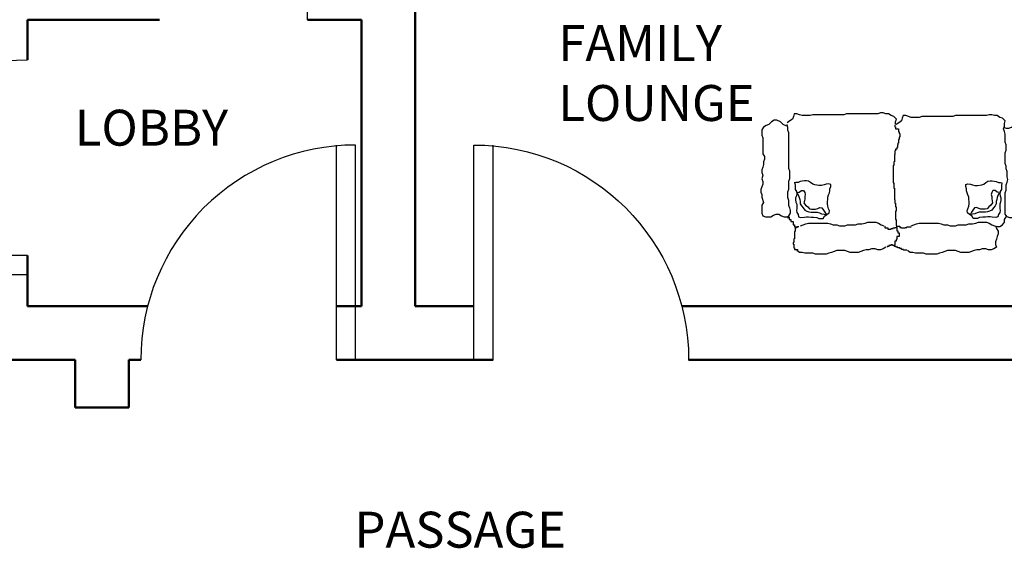
# Model space of a CAD drawing. Units: millimetres. Extents: x -857 to 54106, y -13666 to 13947.
# Tile 19 of 41: x 24413 to 28540, y 8565 to 10779. Entities that reach past the tile are written whole.
import ezdxf

# ---------------------------------------------------------------- set-up
doc = ezdxf.new("R2010")
doc.units = ezdxf.units.MM
for name, color, linetype, lineweight in [('A-AREA-IDEN', 3, 'Continuous', 18), ('A-DOOR', 1, 'Continuous', 25), ('A-FURN', 21, 'Continuous', 18), ('A-WALL', 7, 'Continuous', 50)]:
    doc.layers.add(name, color=color, linetype=linetype, lineweight=lineweight)
doc.layers.add('TEFRIŞ', color=11, linetype='Continuous')
doc.styles.get("Standard").update_dxf_attribs({"font": 'arial.ttf'})

# ---------------------------------------------------------------- blocks, each defined once
blk = doc.blocks.new('26')
at = {"layer": 'TEFRIŞ'}
for p, q in [((-1607.8, -262.65), (-1607.31, -261.17)), ((-1607.31, -261.17), (-1605.84, -261.17)), ((-1605.84, -261.17), (-1604.36, -261.66)), ((-1604.36, -261.66), (-1602.88, -261.66)), ((-1602.88, -261.66), (-1601.41, -262.16)), ((-1591.08, -262.16), (-1589.6, -261.66)), ((-1589.6, -261.66), (-1588.12, -260.68)), ((-1588.12, -260.68), (-1586.16, -260.68)), ((-1586.16, -260.68), (-1584.68, -261.17)), ((-1584.68, -261.17), (-1583.21, -261.66)), ((-1583.21, -261.66), (-1581.73, -261.66)), ((-1581.73, -261.66), (-1580.25, -261.17)), ((-1580.25, -261.17), (-1577.3, -261.17)), ((-1577.3, -261.17), (-1575.83, -260.68)), ((-1575.83, -260.68), (-1572.87, -260.68)), ((-1572.87, -260.68), (-1571.4, -261.17)), ((-1571.4, -261.17), (-1568.45, -261.17)), ((-1568.45, -261.17), (-1566.97, -260.68)), ((-1566.97, -260.68), (-1564.02, -260.68)), ((-1564.02, -260.68), (-1561.07, -261.66)), ((-1561.07, -261.66), (-1559.59, -261.66)), ((-1559.59, -261.66), (-1558.61, -263.14)), ((-1609.77, -265.11), (-1609.28, -263.63)), ((-1609.77, -271.02), (-1609.77, -265.11)), ((-1609.28, -263.63), (-1607.8, -262.65)), ((-1601.41, -262.16), (-1596.98, -262.16)), ((-1596.98, -262.16), (-1595.5, -262.65)), ((-1595.5, -262.65), (-1594.03, -263.63)), ((-1594.03, -263.63), (-1592.55, -262.65)), ((-1592.55, -262.65), (-1591.08, -262.16)), ((-1558.12, -264.62), (-1559.1, -266.1)), ((-1559.1, -266.1), (-1559.1, -270.03)), ((-1558.61, -263.14), (-1558.12, -264.62)), ((-1609.28, -272.49), (-1609.77, -271.02)), ((-1608.29, -273.97), (-1609.28, -272.49)), ((-1559.1, -270.03), (-1558.61, -271.51)), ((-1558.61, -271.51), (-1558.12, -272.99)), ((-1611.74, -277.42), (-1613.21, -278.89)), ((-1610.26, -277.91), (-1611.74, -277.42)), ((-1608.79, -277.91), (-1610.26, -277.91)), ((-1607.31, -278.4), (-1608.79, -277.91)), ((-1607.8, -275.45), (-1608.29, -273.97)), ((-1608.29, -278.4), (-1607.8, -276.93)), ((-1607.8, -276.93), (-1607.8, -275.45)), ((-1605.84, -277.91), (-1607.31, -278.4)), ((-1604.36, -277.42), (-1605.84, -277.91)), ((-1599.93, -277.42), (-1604.36, -277.42)), ((-1598.46, -276.93), (-1599.93, -277.42)), ((-1595.5, -276.93), (-1598.46, -276.93)), ((-1594.03, -277.42), (-1595.5, -276.93)), ((-1588.12, -277.42), (-1594.03, -277.42)), ((-1586.65, -276.93), (-1588.12, -277.42)), ((-1585.17, -276.93), (-1586.65, -276.93)), ((-1583.7, -276.43), (-1585.17, -276.93)), ((-1580.75, -276.43), (-1583.7, -276.43)), ((-1579.27, -275.94), (-1580.75, -276.43)), ((-1577.79, -276.43), (-1579.27, -275.94)), ((-1576.32, -276.93), (-1577.79, -276.43)), ((-1573.37, -276.93), (-1576.32, -276.93)), ((-1571.89, -277.42), (-1573.37, -276.93)), ((-1560.08, -277.42), (-1571.89, -277.42)), ((-1558.61, -276.43), (-1560.08, -277.42)), ((-1558.12, -274.96), (-1558.61, -276.43)), ((-1557.13, -277.91), (-1558.61, -276.93)), ((-1558.12, -272.99), (-1558.12, -274.96)), ((-1555.66, -277.91), (-1557.13, -277.91)), ((-1554.18, -278.89), (-1555.66, -277.91)), ((-1614.69, -283.33), (-1615.18, -284.8)), ((-1613.71, -280.37), (-1614.69, -281.85)), ((-1614.69, -281.85), (-1614.69, -283.33)), ((-1613.21, -278.89), (-1613.71, -280.37)), ((-1578.62, -284.68), (-1578.39, -283.52)), ((-1578.39, -283.52), (-1578.16, -282.36)), ((-1578.16, -282.36), (-1577.69, -281.2)), ((-1577.69, -280.04), (-1577.46, -279.11)), ((-1577.69, -281.2), (-1577.69, -280.04)), ((-1577.23, -279.34), (-1576.07, -279.57)), ((-1576.07, -279.57), (-1573.75, -279.57)), ((-1573.75, -279.57), (-1572.59, -280.27)), ((-1572.36, -281.89), (-1573.29, -283.05)), ((-1573.29, -283.05), (-1573.29, -284.21)), ((-1572.59, -280.27), (-1571.43, -280.5)), ((-1572.13, -280.73), (-1572.36, -281.89)), ((-1571.66, -280.73), (-1570.51, -281.43)), ((-1571.43, -280.5), (-1570.27, -280.27)), ((-1570.51, -281.43), (-1569.35, -281.89)), ((-1570.27, -280.27), (-1569.12, -279.81)), ((-1569.35, -281.89), (-1568.19, -282.13)), ((-1569.12, -279.81), (-1567.96, -279.81)), ((-1568.19, -282.13), (-1567.03, -282.36)), ((-1567.96, -279.81), (-1566.8, -280.04)), ((-1567.03, -282.36), (-1565.87, -282.36)), ((-1566.8, -280.04), (-1565.64, -280.5)), ((-1565.87, -282.36), (-1564.71, -283.05)), ((-1565.64, -280.5), (-1563.32, -280.5)), ((-1564.71, -283.05), (-1563.55, -283.98)), ((-1563.32, -280.5), (-1562.16, -280.27)), ((-1562.16, -280.27), (-1561, -280.5)), ((-1561, -280.5), (-1559.84, -281.2)), ((-1559.84, -281.2), (-1558.68, -281.43)), ((-1558.68, -281.43), (-1558.22, -282.59)), ((-1558.22, -282.59), (-1558.45, -284.68)), ((-1553.2, -280.37), (-1554.18, -278.89)), ((-1554.18, -284.8), (-1553.69, -283.33)), ((-1553.69, -283.33), (-1553.2, -281.85)), ((-1553.69, -282.83), (-1552.21, -282.34)), ((-1553.2, -281.85), (-1553.2, -280.37)), ((-1552.21, -282.34), (-1550.74, -281.36)), ((-1550.74, -281.36), (-1549.26, -281.36)), ((-1549.26, -281.36), (-1547.78, -281.85)), ((-1547.78, -281.85), (-1546.31, -282.34)), ((-1546.31, -282.34), (-1544.83, -282.83)), ((-1544.83, -282.83), (-1543.36, -282.83)), ((-1543.36, -282.83), (-1541.88, -282.34)), ((-1541.88, -282.34), (-1540.9, -283.82)), ((-1540.9, -283.82), (-1540.4, -285.29)), ((-1615.18, -284.8), (-1615.18, -286.28)), ((-1615.18, -286.28), (-1614.69, -287.76)), ((-1614.69, -287.76), (-1614.69, -304.99)), ((-1578.62, -285.84), (-1578.62, -284.68)), ((-1578.39, -287), (-1578.62, -285.84)), ((-1577.69, -288.16), (-1578.39, -287)), ((-1576.76, -289.32), (-1577.69, -288.16)), ((-1576.3, -290.48), (-1576.76, -289.32)), ((-1573.29, -284.21), (-1572.13, -284.91)), ((-1572.13, -284.91), (-1570.97, -285.14)), ((-1570.97, -285.14), (-1569.81, -284.91)), ((-1569.81, -284.91), (-1568.65, -284.91)), ((-1568.65, -284.91), (-1567.49, -284.68)), ((-1567.49, -284.68), (-1566.33, -284.45)), ((-1566.33, -284.45), (-1565.17, -285.37)), ((-1565.17, -285.37), (-1564.25, -286.53)), ((-1564.25, -286.53), (-1563.09, -287.46)), ((-1563.55, -283.98), (-1562.39, -284.91)), ((-1563.09, -287.46), (-1562.86, -288.62)), ((-1562.86, -288.62), (-1562.86, -290.94)), ((-1562.39, -284.91), (-1561.7, -286.07)), ((-1561.7, -286.07), (-1561.47, -287.23)), ((-1561.47, -287.23), (-1561.23, -288.39)), ((-1561.23, -288.39), (-1561.23, -291.87)), ((-1558.45, -284.68), (-1558.68, -285.84)), ((-1558.68, -285.84), (-1558.68, -287)), ((-1558.68, -287), (-1558.45, -288.39)), ((-1558.45, -288.39), (-1558.45, -289.78)), ((-1555.66, -287.76), (-1555.16, -286.28)), ((-1555.66, -292.19), (-1555.66, -287.76)), ((-1555.16, -286.28), (-1554.18, -284.8)), ((-1540.4, -286.77), (-1540.9, -288.25)), ((-1540.9, -288.25), (-1540.9, -290.22)), ((-1540.4, -285.29), (-1540.4, -286.77)), ((-1576.07, -292.8), (-1576.3, -290.48)), ((-1576.3, -295.58), (-1576.07, -294.19)), ((-1576.07, -294.19), (-1576.07, -292.8)), ((-1563.32, -292.1), (-1563.78, -293.26)), ((-1563.78, -293.26), (-1563.55, -294.42)), ((-1563.55, -294.42), (-1562.39, -295.35)), ((-1562.86, -290.94), (-1563.32, -292.1)), ((-1561.23, -291.87), (-1560.77, -293.03)), ((-1560.77, -293.03), (-1560.31, -294.19)), ((-1560.31, -294.19), (-1560.07, -295.58)), ((-1558.45, -289.78), (-1558.22, -291.64)), ((-1558.22, -291.64), (-1557.76, -292.8)), ((-1557.76, -292.8), (-1557.76, -295.12)), ((-1555.16, -293.66), (-1555.66, -292.19)), ((-1554.67, -295.63), (-1555.16, -293.66)), ((-1540.9, -290.22), (-1540.4, -291.69)), ((-1540.4, -291.69), (-1540.4, -293.17)), ((-1540.4, -293.17), (-1539.91, -294.65)), ((-1539.91, -294.65), (-1539.42, -296.12)), ((-1577, -298.13), (-1576.76, -296.74)), ((-1576.53, -299.29), (-1577, -298.13)), ((-1576.76, -296.74), (-1576.3, -295.58)), ((-1575.37, -299.29), (-1576.53, -299.29)), ((-1574.21, -298.83), (-1575.37, -299.29)), ((-1573.06, -298.83), (-1574.21, -298.83)), ((-1571.9, -298.59), (-1573.06, -298.83)), ((-1570.74, -298.13), (-1571.9, -298.59)), ((-1569.58, -297.67), (-1570.74, -298.13)), ((-1568.19, -297.67), (-1569.58, -297.67)), ((-1567.03, -297.43), (-1568.19, -297.67)), ((-1565.87, -297.43), (-1567.03, -297.43)), ((-1564.48, -297.67), (-1565.87, -297.43)), ((-1563.09, -298.13), (-1564.48, -297.67)), ((-1561.93, -298.59), (-1563.09, -298.13)), ((-1562.39, -295.35), (-1561.23, -296.04)), ((-1560.77, -298.36), (-1561.93, -298.59)), ((-1561.23, -296.04), (-1560.07, -296.74)), ((-1559.84, -297.2), (-1560.77, -298.36)), ((-1560.07, -295.58), (-1559.84, -296.74)), ((-1560.07, -296.74), (-1559.61, -296.97)), ((-1558.92, -295.81), (-1559.84, -297.2)), ((-1557.76, -295.12), (-1558.92, -295.81)), ((-1554.67, -297.6), (-1554.67, -295.63)), ((-1554.18, -299.08), (-1554.67, -297.6)), ((-1554.18, -303.51), (-1554.18, -299.08)), ((-1539.42, -296.12), (-1538.93, -297.6)), ((-1538.93, -297.6), (-1538.93, -302.03)), ((-1614.69, -304.99), (-1614.2, -306.46)), ((-1553.69, -304.99), (-1554.18, -303.51)), ((-1553.69, -307.94), (-1553.69, -304.99)), ((-1539.42, -303.51), (-1539.91, -304.99)), ((-1539.91, -304.99), (-1539.91, -309.42)), ((-1538.93, -302.03), (-1539.42, -303.51)), ((-1614.2, -306.46), (-1614.2, -323.69)), ((-1554.18, -309.42), (-1553.69, -307.94)), ((-1554.18, -311.39), (-1554.18, -309.42)), ((-1539.91, -309.42), (-1539.42, -310.89)), ((-1539.42, -310.89), (-1538.93, -312.37)), ((-1555.16, -314.34), (-1554.67, -312.86)), ((-1555.16, -325.17), (-1555.16, -314.34)), ((-1554.67, -312.86), (-1554.18, -311.39)), ((-1538.93, -312.37), (-1538.44, -313.85)), ((-1538.44, -313.85), (-1537.95, -315.32)), ((-1537.95, -315.32), (-1537.95, -321.23)), ((-1537.95, -321.23), (-1538.44, -322.71)), ((-1614.2, -323.69), (-1613.71, -325.17)), ((-1613.71, -325.17), (-1613.71, -329.6)), ((-1554.67, -326.65), (-1555.16, -325.17)), ((-1554.18, -328.12), (-1554.67, -326.65)), ((-1538.44, -327.14), (-1538.93, -328.62)), ((-1538.44, -322.71), (-1538.44, -327.14)), ((-1614.2, -331.08), (-1614.69, -332.55)), ((-1614.69, -332.55), (-1614.69, -334.03)), ((-1613.71, -329.6), (-1614.2, -331.08)), ((-1553.69, -329.6), (-1554.18, -328.12)), ((-1553.13, -331.91), (-1553.13, -329.57)), ((-1552.79, -331.91), (-1553.13, -331.91)), ((-1552.79, -332.91), (-1552.79, -331.91)), ((-1552.46, -332.91), (-1552.79, -332.91)), ((-1552.46, -334.91), (-1552.46, -332.91)), ((-1540.13, -331.91), (-1540.13, -333.91)), ((-1538.93, -330.09), (-1539.91, -331.57)), ((-1538.93, -328.62), (-1538.93, -330.09)), ((-1614.69, -334.03), (-1613.21, -334.52)), ((-1612.74, -337.78), (-1614.21, -339.26)), ((-1613.21, -334.52), (-1611.74, -335.02)), ((-1611.26, -338.27), (-1612.74, -337.78)), ((-1611.74, -335.02), (-1610.75, -336.49)), ((-1609.79, -338.27), (-1611.26, -338.27)), ((-1610.75, -336.49), (-1609.77, -337.97)), ((-1608.45, -338.58), (-1608.45, -338.24)), ((-1608.45, -338.24), (-1607.45, -338.24)), ((-1607.45, -338.24), (-1607.45, -336.58)), ((-1607.45, -336.58), (-1605.78, -336.58)), ((-1605.78, -336.58), (-1605.78, -336.24)), ((-1605.78, -336.24), (-1604.78, -336.24)), ((-1604.78, -336.24), (-1604.78, -335.91)), ((-1604.78, -335.91), (-1602.79, -335.91)), ((-1602.79, -335.91), (-1602.79, -336.24)), ((-1602.79, -336.24), (-1601.45, -336.24)), ((-1601.45, -336.24), (-1601.45, -336.58)), ((-1601.45, -336.58), (-1599.45, -336.58)), ((-1599.45, -336.58), (-1599.45, -336.91)), ((-1599.45, -336.91), (-1598.45, -336.91)), ((-1598.45, -336.91), (-1598.45, -337.24)), ((-1598.45, -337.24), (-1597.12, -337.24)), ((-1597.12, -337.24), (-1597.12, -337.58)), ((-1597.12, -337.58), (-1596.12, -337.58)), ((-1596.12, -337.58), (-1596.12, -338.24)), ((-1596.12, -338.24), (-1595.12, -338.24)), ((-1595.12, -338.24), (-1595.12, -338.58)), ((-1566.13, -338.58), (-1566.13, -338.24)), ((-1566.13, -338.24), (-1564.13, -338.24)), ((-1564.13, -338.24), (-1564.13, -337.91)), ((-1564.13, -337.91), (-1561.79, -337.91)), ((-1561.79, -337.91), (-1561.79, -338.24)), ((-1561.79, -338.24), (-1557.13, -338.24)), ((-1557.13, -338.24), (-1557.13, -337.91)), ((-1557.13, -337.91), (-1553.79, -337.91)), ((-1553.79, -337.91), (-1553.79, -337.58)), ((-1553.46, -337.91), (-1553.46, -335.91)), ((-1553.46, -335.91), (-1552.79, -335.91)), ((-1552.79, -337.58), (-1553.13, -337.58)), ((-1553.13, -337.58), (-1553.13, -337.91)), ((-1552.79, -335.91), (-1552.79, -334.91)), ((-1552.79, -334.91), (-1552.46, -334.91)), ((-1552.79, -338.58), (-1552.79, -337.58)), ((-1552.79, -337.58), (-1550.8, -337.58)), ((-1550.8, -337.58), (-1550.8, -336.91)), ((-1550.8, -336.91), (-1549.8, -336.91)), ((-1549.8, -336.91), (-1549.8, -336.24)), ((-1549.8, -336.24), (-1547.8, -336.24)), ((-1547.8, -336.24), (-1547.8, -337.58)), ((-1547.8, -337.58), (-1546.13, -337.58)), ((-1546.13, -337.58), (-1546.13, -337.91)), ((-1546.13, -337.91), (-1545.13, -337.91)), ((-1545.13, -337.91), (-1545.13, -338.58)), ((-1541.8, -337.91), (-1542.13, -337.91)), ((-1542.13, -337.91), (-1542.13, -338.91)), ((-1541.46, -336.91), (-1541.8, -336.91)), ((-1541.8, -336.91), (-1541.8, -337.91)), ((-1541.13, -335.91), (-1541.46, -335.91)), ((-1541.46, -335.91), (-1541.46, -336.91)), ((-1540.46, -334.91), (-1541.13, -334.91)), ((-1541.13, -334.91), (-1541.13, -335.91)), ((-1540.13, -333.91), (-1540.46, -333.91)), ((-1540.46, -333.91), (-1540.46, -334.91)), ((-1615.69, -343.69), (-1616.18, -345.16)), ((-1614.71, -340.73), (-1615.69, -342.21)), ((-1615.69, -342.21), (-1615.69, -343.69)), ((-1614.21, -339.26), (-1614.71, -340.73)), ((-1609.45, -338.58), (-1608.45, -338.58)), ((-1595.12, -338.58), (-1593.12, -338.58)), ((-1593.12, -338.58), (-1593.12, -338.91)), ((-1593.12, -338.91), (-1589.12, -338.91)), ((-1589.12, -338.91), (-1589.12, -339.25)), ((-1589.12, -339.25), (-1587.12, -339.25)), ((-1587.12, -339.25), (-1587.12, -339.58)), ((-1587.12, -339.58), (-1577.46, -339.58)), ((-1577.46, -339.58), (-1577.46, -339.25)), ((-1577.46, -339.25), (-1574.46, -339.25)), ((-1574.46, -339.25), (-1574.46, -338.91)), ((-1574.46, -338.91), (-1568.13, -338.91)), ((-1568.13, -338.91), (-1568.13, -338.58)), ((-1568.13, -338.58), (-1566.13, -338.58)), ((-1552.46, -338.58), (-1552.79, -338.58)), ((-1552.46, -339.58), (-1552.46, -338.58)), ((-1552.13, -339.58), (-1552.46, -339.58)), ((-1552.46, -344.25), (-1552.46, -342.58)), ((-1552.46, -342.58), (-1551.8, -342.58)), ((-1552.13, -340.58), (-1552.13, -339.58)), ((-1551.8, -340.58), (-1552.13, -340.58)), ((-1551.8, -342.58), (-1551.8, -340.58)), ((-1545.13, -338.58), (-1543.13, -338.58)), ((-1543.13, -338.58), (-1543.13, -338.91)), ((-1543.13, -338.91), (-1542.8, -338.91)), ((-1542.8, -339.91), (-1543.13, -339.91)), ((-1543.13, -339.91), (-1543.13, -340.91)), ((-1543.13, -340.91), (-1542.8, -340.91)), ((-1542.13, -338.91), (-1542.8, -338.91)), ((-1542.8, -338.91), (-1542.8, -339.91)), ((-1542.8, -340.91), (-1542.8, -341.91)), ((-1542.8, -341.91), (-1542.13, -341.91)), ((-1542.13, -341.91), (-1542.13, -342.91)), ((-1542.13, -342.91), (-1541.8, -342.91)), ((-1541.88, -343.7), (-1540.9, -345.18)), ((-1616.18, -345.16), (-1616.18, -346.64)), ((-1616.18, -346.64), (-1615.69, -348.12)), ((-1615.69, -348.12), (-1615.69, -365.35)), ((-1555.66, -349.12), (-1555.16, -347.64)), ((-1555.66, -353.55), (-1555.66, -349.12)), ((-1555.16, -347.64), (-1554.18, -346.17)), ((-1554.18, -346.17), (-1553.69, -344.69)), ((-1553.46, -344.25), (-1552.46, -344.25)), ((-1540.9, -345.18), (-1540.4, -346.66)), ((-1540.4, -348.13), (-1540.9, -349.61)), ((-1540.4, -346.66), (-1540.4, -348.13)), ((-1555.16, -355.03), (-1555.66, -353.55)), ((-1540.9, -349.61), (-1540.9, -351.58)), ((-1540.9, -351.58), (-1540.4, -353.06)), ((-1540.4, -353.06), (-1540.4, -354.53)), ((-1540.4, -354.53), (-1539.91, -356.01)), ((-1554.67, -357), (-1555.16, -355.03)), ((-1554.67, -358.96), (-1554.67, -357)), ((-1554.18, -360.44), (-1554.67, -358.96)), ((-1539.91, -356.01), (-1539.42, -357.49)), ((-1539.42, -357.49), (-1538.93, -358.96)), ((-1538.93, -358.96), (-1538.93, -363.4)), ((-1615.69, -365.35), (-1615.2, -366.83)), ((-1554.18, -364.87), (-1554.18, -360.44)), ((-1553.69, -366.35), (-1554.18, -364.87)), ((-1539.42, -364.87), (-1539.91, -366.35)), ((-1538.93, -363.4), (-1539.42, -364.87)), ((-1615.2, -366.83), (-1615.2, -384.06)), ((-1554.18, -370.78), (-1553.69, -369.3)), ((-1554.18, -372.75), (-1554.18, -370.78)), ((-1553.69, -369.3), (-1553.69, -366.35)), ((-1539.91, -366.35), (-1539.91, -370.78)), ((-1539.91, -370.78), (-1539.42, -372.26)), ((-1576.53, -374.2), (-1577, -375.36)), ((-1577, -375.36), (-1576.76, -376.75)), ((-1575.37, -374.2), (-1576.53, -374.2)), ((-1574.21, -374.66), (-1575.37, -374.2)), ((-1573.06, -374.66), (-1574.21, -374.66)), ((-1571.9, -374.89), (-1573.06, -374.66)), ((-1570.74, -375.36), (-1571.9, -374.89)), ((-1569.58, -375.82), (-1570.74, -375.36)), ((-1568.19, -375.82), (-1569.58, -375.82)), ((-1567.03, -376.05), (-1568.19, -375.82)), ((-1565.87, -376.05), (-1567.03, -376.05)), ((-1564.48, -375.82), (-1565.87, -376.05)), ((-1563.09, -375.36), (-1564.48, -375.82)), ((-1561.93, -374.89), (-1563.09, -375.36)), ((-1560.77, -375.12), (-1561.93, -374.89)), ((-1559.84, -376.28), (-1560.77, -375.12)), ((-1560.07, -376.75), (-1559.61, -376.52)), ((-1558.92, -377.68), (-1559.84, -376.28)), ((-1555.16, -375.7), (-1554.67, -374.23)), ((-1555.16, -386.53), (-1555.16, -375.7)), ((-1554.67, -374.23), (-1554.18, -372.75)), ((-1539.42, -372.26), (-1538.93, -373.73)), ((-1538.93, -373.73), (-1538.44, -375.21)), ((-1538.44, -375.21), (-1537.95, -376.69)), ((-1537.95, -376.69), (-1537.95, -382.59)), ((-1576.76, -376.75), (-1576.3, -377.91)), ((-1576.3, -377.91), (-1576.07, -379.3)), ((-1576.07, -380.69), (-1576.3, -383.01)), ((-1576.07, -379.3), (-1576.07, -380.69)), ((-1563.78, -380.23), (-1563.55, -379.07)), ((-1563.32, -381.39), (-1563.78, -380.23)), ((-1563.55, -379.07), (-1562.39, -378.14)), ((-1562.86, -382.55), (-1563.32, -381.39)), ((-1562.39, -378.14), (-1561.23, -377.44)), ((-1561.23, -377.44), (-1560.07, -376.75)), ((-1561.23, -381.62), (-1560.77, -380.46)), ((-1561.23, -385.1), (-1561.23, -381.62)), ((-1560.77, -380.46), (-1560.31, -379.3)), ((-1560.31, -379.3), (-1560.07, -377.91)), ((-1560.07, -377.91), (-1559.84, -376.75)), ((-1557.76, -378.37), (-1558.92, -377.68)), ((-1558.45, -383.71), (-1558.22, -381.85)), ((-1558.22, -381.85), (-1557.76, -380.69)), ((-1557.76, -380.69), (-1557.76, -378.37)), ((-1615.2, -384.06), (-1614.71, -385.53)), ((-1614.71, -385.53), (-1614.71, -389.96)), ((-1578.39, -386.49), (-1578.62, -387.65)), ((-1577.69, -385.33), (-1578.39, -386.49)), ((-1576.76, -384.17), (-1577.69, -385.33)), ((-1576.3, -383.01), (-1576.76, -384.17)), ((-1565.17, -388.11), (-1564.25, -386.95)), ((-1564.25, -386.95), (-1563.09, -386.03)), ((-1563.09, -386.03), (-1562.86, -384.87)), ((-1562.86, -384.87), (-1562.86, -382.55)), ((-1562.39, -388.58), (-1561.7, -387.42)), ((-1561.7, -387.42), (-1561.47, -386.26)), ((-1561.47, -386.26), (-1561.23, -385.1)), ((-1558.68, -386.49), (-1558.45, -385.1)), ((-1558.68, -387.65), (-1558.68, -386.49)), ((-1558.45, -385.1), (-1558.45, -383.71)), ((-1554.67, -388.01), (-1555.16, -386.53)), ((-1537.95, -382.59), (-1538.44, -384.07)), ((-1538.44, -384.07), (-1538.44, -388.5)), ((-1615.2, -391.44), (-1615.69, -392.92)), ((-1615.69, -392.92), (-1615.69, -394.39)), ((-1614.71, -389.96), (-1615.2, -391.44)), ((-1578.62, -387.65), (-1578.62, -388.81)), ((-1578.62, -388.81), (-1578.39, -389.97)), ((-1578.39, -389.97), (-1578.16, -391.13)), ((-1578.16, -391.13), (-1577.69, -392.29)), ((-1577.69, -392.29), (-1577.69, -393.45)), ((-1573.29, -389.27), (-1572.13, -388.58)), ((-1573.29, -390.43), (-1573.29, -389.27)), ((-1572.36, -391.59), (-1573.29, -390.43)), ((-1572.59, -393.22), (-1571.43, -392.99)), ((-1572.13, -392.75), (-1572.36, -391.59)), ((-1572.13, -388.58), (-1570.97, -388.35)), ((-1571.66, -392.75), (-1570.51, -392.06)), ((-1571.43, -392.99), (-1570.27, -393.22)), ((-1570.97, -388.35), (-1569.81, -388.58)), ((-1570.51, -392.06), (-1569.35, -391.59)), ((-1569.81, -388.58), (-1568.65, -388.58)), ((-1569.35, -391.59), (-1568.19, -391.36)), ((-1568.65, -388.58), (-1567.49, -388.81)), ((-1568.19, -391.36), (-1567.03, -391.13)), ((-1567.49, -388.81), (-1566.33, -389.04)), ((-1567.03, -391.13), (-1565.87, -391.13)), ((-1566.8, -393.45), (-1565.64, -392.99)), ((-1566.33, -389.04), (-1565.17, -388.11)), ((-1565.87, -391.13), (-1564.71, -390.43)), ((-1565.64, -392.99), (-1563.32, -392.99)), ((-1564.71, -390.43), (-1563.55, -389.51)), ((-1563.55, -389.51), (-1562.39, -388.58)), ((-1563.32, -392.99), (-1562.16, -393.22)), ((-1562.16, -393.22), (-1561, -392.99)), ((-1561, -392.99), (-1559.84, -392.29)), ((-1559.84, -392.29), (-1558.68, -392.06)), ((-1558.45, -388.81), (-1558.68, -387.65)), ((-1558.68, -392.06), (-1558.22, -390.9)), ((-1558.22, -390.9), (-1558.45, -388.81)), ((-1554.18, -389.49), (-1554.67, -388.01)), ((-1553.69, -390.96), (-1554.18, -389.49)), ((-1553.13, -391.94), (-1553.13, -392.94)), ((-1553.13, -392.94), (-1552.46, -392.94)), ((-1552.46, -392.94), (-1552.46, -393.94)), ((-1540.46, -394.27), (-1540.46, -392.6)), ((-1540.46, -392.6), (-1539.8, -392.6)), ((-1538.93, -391.46), (-1539.91, -392.93)), ((-1538.44, -388.5), (-1538.93, -389.98)), ((-1538.93, -389.98), (-1538.93, -391.46)), ((-1615.69, -394.39), (-1614.21, -394.89)), ((-1614.21, -394.89), (-1612.74, -395.38)), ((-1612.74, -395.38), (-1611.75, -396.85)), ((-1611.75, -396.85), (-1610.77, -398.33)), ((-1609.77, -398.57), (-1608.29, -398.08)), ((-1608.29, -398.08), (-1606.82, -398.08)), ((-1606.82, -398.08), (-1605.34, -397.59)), ((-1605.34, -397.59), (-1585.66, -397.59)), ((-1585.66, -397.59), (-1584.19, -397.1)), ((-1584.19, -397.1), (-1579.76, -397.1)), ((-1579.76, -397.1), (-1578.29, -397.59)), ((-1578.29, -397.59), (-1573.86, -397.59)), ((-1577.69, -393.45), (-1577.46, -394.38)), ((-1577.23, -394.15), (-1576.07, -393.91)), ((-1576.07, -393.91), (-1573.75, -393.91)), ((-1573.86, -397.59), (-1572.38, -398.08)), ((-1573.75, -393.91), (-1572.59, -393.22)), ((-1572.38, -398.08), (-1569.43, -398.08)), ((-1570.27, -393.22), (-1569.12, -393.68)), ((-1569.43, -398.08), (-1567.95, -397.59)), ((-1569.12, -393.68), (-1567.96, -393.68)), ((-1567.96, -393.68), (-1566.8, -393.45)), ((-1567.95, -397.59), (-1565, -397.59)), ((-1565, -397.59), (-1563.53, -397.1)), ((-1563.53, -397.1), (-1562.05, -396.6)), ((-1562.05, -396.6), (-1560.58, -396.6)), ((-1560.58, -396.6), (-1559.1, -397.59)), ((-1558.61, -398.57), (-1559.1, -397.1)), ((-1559.1, -397.59), (-1557.62, -398.08)), ((-1558.46, -397.27), (-1557.13, -397.27)), ((-1557.13, -397.27), (-1557.13, -396.27)), ((-1557.13, -396.27), (-1556.13, -396.27)), ((-1556.13, -396.27), (-1556.13, -394.94)), ((-1556.13, -394.94), (-1554.13, -394.94)), ((-1554.13, -394.94), (-1554.13, -394.27)), ((-1554.13, -394.27), (-1553.13, -394.27)), ((-1553.13, -394.27), (-1553.13, -393.27)), ((-1553.13, -393.27), (-1552.46, -393.27)), ((-1552.46, -393.94), (-1550.46, -393.94)), ((-1550.46, -393.94), (-1550.46, -394.27)), ((-1550.46, -394.27), (-1546.46, -394.27)), ((-1546.46, -394.27), (-1546.46, -394.61)), ((-1546.46, -394.61), (-1544.46, -394.61)), ((-1544.46, -394.61), (-1544.46, -394.94)), ((-1544.46, -394.94), (-1543.46, -394.94)), ((-1543.46, -394.94), (-1543.46, -394.61)), ((-1543.46, -394.61), (-1541.46, -394.61)), ((-1541.46, -394.61), (-1541.46, -394.27)), ((-1541.46, -394.27), (-1540.46, -394.27)), ((-1611.25, -402.02), (-1612.23, -403.99)), ((-1612.23, -403.99), (-1612.23, -405.47)), ((-1609.77, -400.54), (-1611.25, -402.02)), ((-1608.79, -398.57), (-1609.77, -400.54)), ((-1560.08, -403), (-1559.1, -401.53)), ((-1560.08, -404.48), (-1560.08, -403)), ((-1559.1, -401.53), (-1558.61, -400.05)), ((-1558.61, -400.05), (-1558.61, -398.57)), ((-1612.23, -405.47), (-1611.25, -406.94)), ((-1611.25, -406.94), (-1609.77, -408.42)), ((-1609.77, -408.42), (-1609.28, -409.9)), ((-1559.59, -405.96), (-1560.08, -404.48)), ((-1558.61, -407.43), (-1559.59, -405.96)), ((-1558.61, -410.39), (-1558.61, -407.43)), ((-1609.28, -409.9), (-1608.29, -411.37)), ((-1608.29, -411.37), (-1606.82, -412.36)), ((-1606.82, -412.36), (-1603.87, -412.36)), ((-1603.87, -412.36), (-1602.39, -411.86)), ((-1602.39, -411.86), (-1593.54, -411.86)), ((-1593.54, -411.86), (-1592.06, -410.88)), ((-1592.06, -410.88), (-1590.58, -410.88)), ((-1590.58, -410.88), (-1589.11, -411.37)), ((-1589.11, -411.37), (-1587.63, -411.37)), ((-1587.63, -411.37), (-1586.16, -411.86)), ((-1586.16, -411.86), (-1584.68, -412.36)), ((-1584.68, -412.36), (-1583.21, -412.36)), ((-1583.21, -412.36), (-1581.73, -411.86)), ((-1581.73, -411.86), (-1579.76, -412.36)), ((-1579.76, -412.36), (-1578.29, -411.86)), ((-1578.29, -411.86), (-1576.81, -411.86)), ((-1576.81, -411.86), (-1575.33, -412.36)), ((-1575.33, -412.36), (-1573.86, -412.85)), ((-1573.86, -412.85), (-1572.38, -412.85)), ((-1572.38, -412.85), (-1570.91, -412.36)), ((-1570.91, -412.36), (-1569.43, -412.36)), ((-1569.43, -412.36), (-1566.48, -411.37)), ((-1566.48, -411.37), (-1565, -412.36)), ((-1565, -412.36), (-1560.58, -412.36)), ((-1560.58, -412.36), (-1559.1, -411.86)), ((-1559.1, -411.86), (-1558.61, -410.39))]:
    blk.add_line(p, q, dxfattribs=at)
blk = doc.blocks.new('DOOR-900')
blk.add_line((11417.3, 9811.5), (12317.3, 9811.5))
blk.add_arc((11417.3, 9811.5), 900, 0, 90)

msp = doc.modelspace()

# ---------------------------------------------------------------- linework, layer by layer
at = {"layer": 'A-DOOR'}
for p, q in [((25618.345, 10779.231), (25618.345, 11479.231)), ((25740.079, 9354.231), (25740.079, 10254.231)), ((26396.59, 9354.231), (26396.59, 10254.231)), ((24445.079, 9791.167), (23545.079, 9791.167))]:
    msp.add_line(p, q, dxfattribs=at)
at = {"layer": 'A-WALL'}
for p, q in [((26070.079, 9579.231), (26070.079, 12579.231)), ((26070.079, 11579.231), (26070.079, 9579.231)), ((24445.079, 10611.167), (24445.079, 10779.231)), ((24445.079, 10779.231), (24998.345, 10779.231)), ((25618.345, 10779.231), (25845.079, 10779.231)), ((25845.079, 10779.231), (25845.079, 9579.231)), ((24445.079, 9579.231), (24445.079, 9791.167)), ((24948.658, 9579.231), (24445.079, 9579.231)), ((25845.079, 9579.231), (25740.079, 9579.231)), ((26070.079, 9579.231), (26316.59, 9579.231)), ((26316.59, 9579.231), (26070.079, 9579.231)), ((29795.079, 9579.231), (27188.012, 9579.231)), ((28170.079, 9579.231), (28870.079, 9579.231)), ((23445.079, 9354.231), (24645.079, 9354.231)), ((24645.079, 9354.231), (24645.079, 9154.231)), ((24870.079, 9354.231), (24870.079, 9154.231)), ((24920.079, 9354.231), (24870.079, 9354.231)), ((26396.59, 9354.231), (25740.079, 9354.231)), ((27216.59, 9354.231), (29820.079, 9354.231)), ((24645.079, 9154.231), (24870.079, 9154.231))]:
    msp.add_line(p, q, dxfattribs=at)

# ---------------------------------------------------------------- block references
at = {"layer": 'A-DOOR', "extrusion": (0, 0, -1), "zscale": -1}
msp.add_blockref('DOOR-900', (-35862.359, -100.315), dxfattribs=at)
at = {"layer": 'A-DOOR', "rotation": 89.99999999999976}
msp.add_blockref('DOOR-900', (35631.56, -2063.049), dxfattribs=at)
at = {"layer": 'A-DOOR', "extrusion": (0, 0, -1), "zscale": -1, "rotation": 90}
msp.add_blockref('DOOR-900', (-16505.109, -2063.049), dxfattribs=at)
at = {"layer": 'A-FURN', "xscale": 7.559220362162901, "yscale": 7.559220362162901, "zscale": 7.559220362162901, "rotation": 270}
msp.add_blockref('26', (30640.69, -1828.483), dxfattribs=at)

# ---------------------------------------------------------------- texts
at = {"layer": 'A-AREA-IDEN', "char_height": 150.48461, "attachment_point": 1}
for s, insert in [('\\pxt0;FAMILY\\PLOUNGE', (26670.476, 10756.437)), ('\\pxt0;LOBBY', (24643.779, 10402.056)), ('\\pxt0;PASSAGE', (25815.869, 8718.225))]:
    msp.add_mtext_dynamic_manual_height_columns(s, width=2554.22693, gutter_width=18810.576, heights=[2595.835], dxfattribs=dict(at, insert=insert))

doc.saveas('drawing.dxf')
